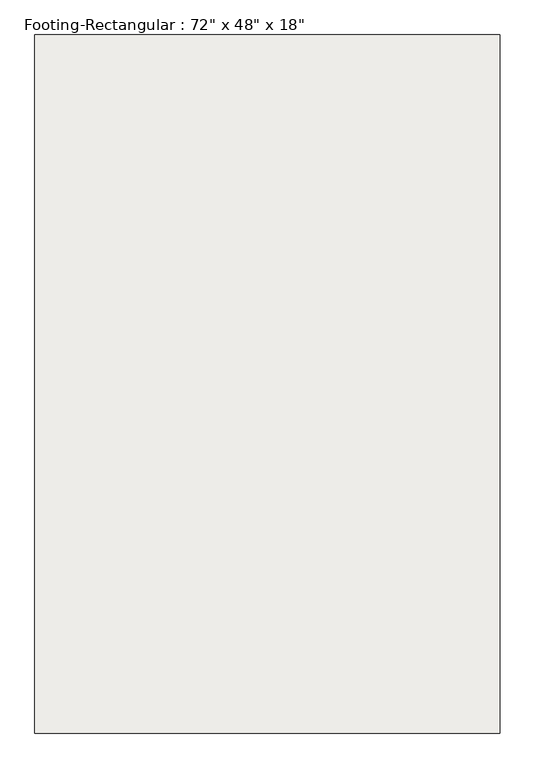
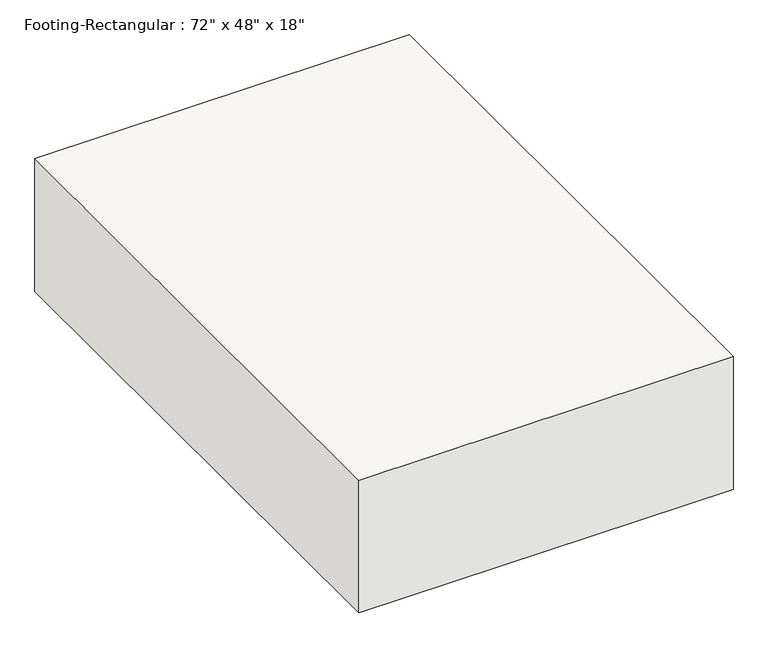
"""IFC4 building model written with IfcOpenShell, lengths in millimetres: slab geometry."""

from ifc_helpers import new_model, si_unit, frame, origin, place, context, project, spatial, polyline, outline, extrude, source, transform, mapped, element, save


def slab_5ba74754(model_context):
    return source(origin(), model_context, "Body", "SweptSolid", [
        extrude(outline(polyline([(609.6, 914.4), (609.6, -914.4), (-609.6, -914.4), (-609.6, 914.4), (609.6, 914.4)])), frame((0.0, 0.0, -457.2), z_axis=(0.0, 0.0, 1.0), x_axis=(1.0, 0.0, 0.0)), (0.0, 0.0, 1.0), 457.2),
    ])


if __name__ == "__main__":
    model = new_model("IFC4")
    model_context = context("Model", 3, world=origin())
    ifc_project = project(units=[si_unit("LENGTHUNIT", "METRE", prefix="MILLI")], contexts=[model_context])
    site = spatial("IfcSite", under=ifc_project)
    building = spatial("IfcBuilding", under=site)
    placement = place(None, origin())
    slab_shape = slab_5ba74754(model_context)
    element("IfcSlab", 1, ObjectType="Footing-Rectangular : 72\" x 48\" x 18\"", at=placement, inside=building, context=model_context, shape_type="MappedRepresentation", body=[
        mapped(slab_shape, transform((0.0, 0.0, 0.0), x_axis=(1.0, 0.0, 0.0), y_axis=(0.0, 1.0, 0.0), z_axis=(0.0, 0.0, 1.0))),
    ])
    save(model, "model.ifc")

# Revit data of these elements
# Type "Footing-Rectangular : 72\" x 48\" x 18\""
#   Assembly Code = "A1010100"
#   Width = 4 ft
#   Length = 6 ft
#   Foundation Thickness = 1.5 ft
#   Structural Material [instance default] = Concrete, Cast-in-Place gray
# Element 1 (IfcSlab, "Footing-Rectangular : 72\" x 48\" x 18\"")
#   Materials on its faces: "Concrete, Cast-in-Place gray"
# Materials
#   "Concrete, Cast-in-Place gray": class "Concrete", colour RGB 192 192 192, transparency 0, Description = "Cast-in-place concrete", Cost = 0
